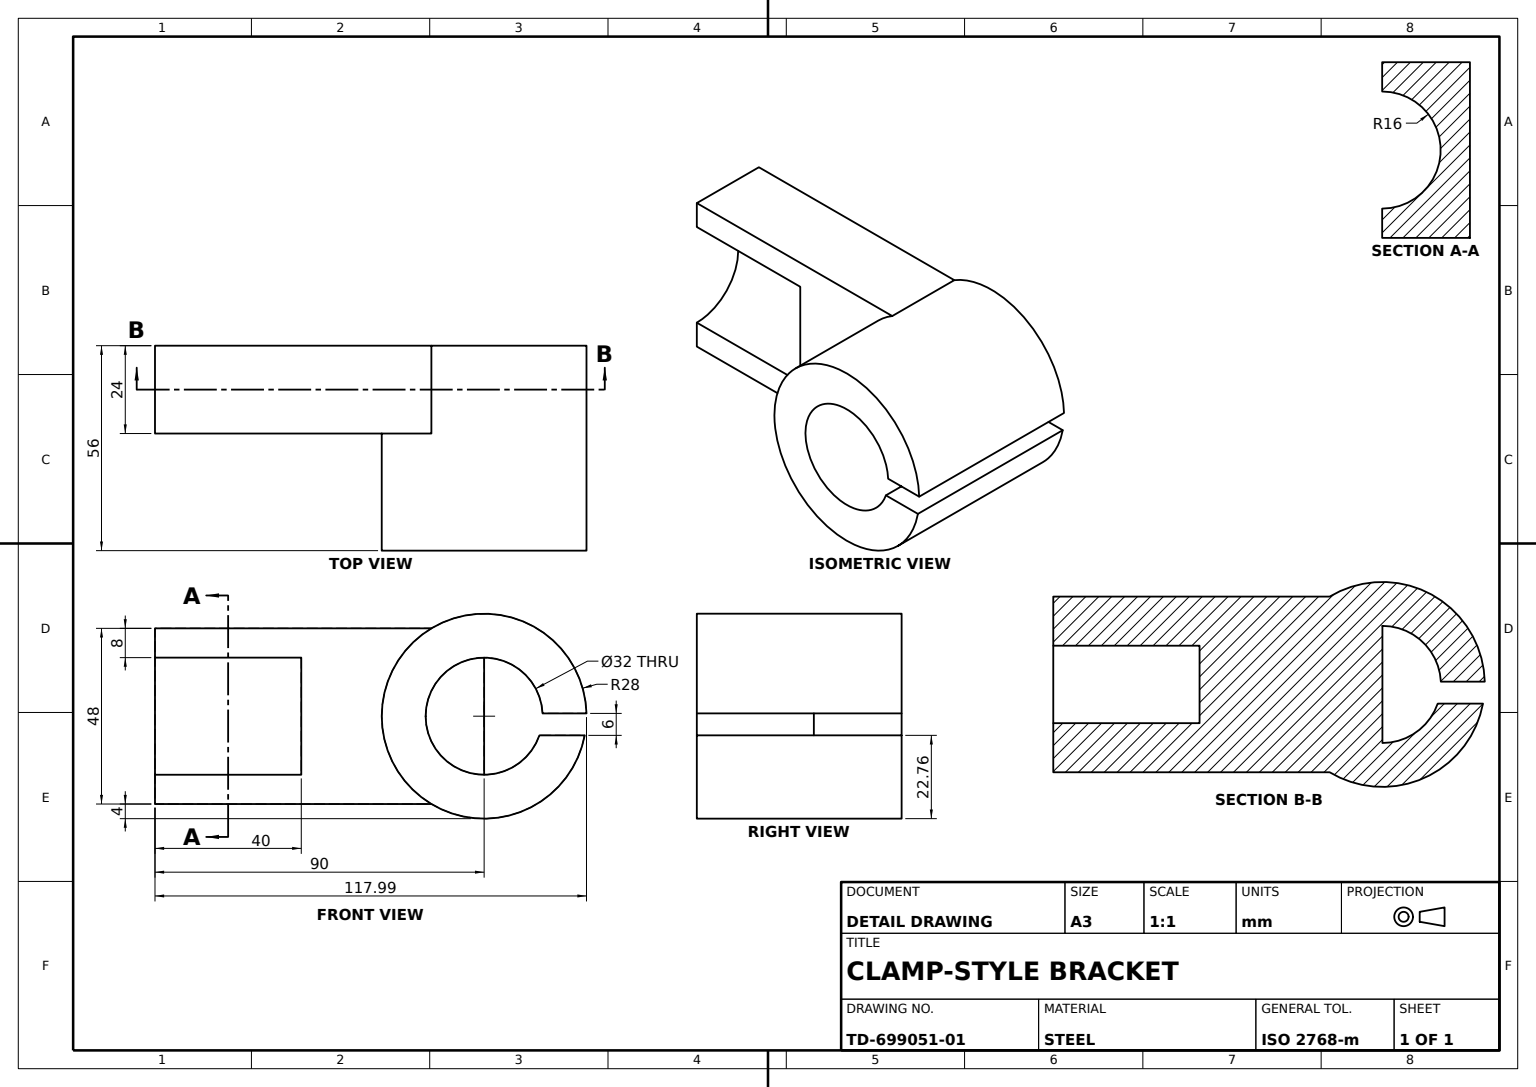
from build123d import *

# Parameters (mm, degrees)
BASE_BLOCK_SKETCH_W           = 90
BASE_BLOCK_SKETCH_H           = 48
BASE_BLOCK_DEPTH              = 12
CRADLE_CUT_DEPTH              = 40
CLAMP_BOSS_SKETCH_R           = 28
CLAMP_BOSS_SKETCH_R_2         = 16
CLAMP_BOSS_56_DEPTH           = 56
BORE_AND_SPLIT_SLOT_CUT_DEPTH = 56


with BuildPart() as part:
    # Base Block Sketch → Base Block (new, symmetric)
    with BuildSketch(Plane.XY):
        Rectangle(BASE_BLOCK_SKETCH_W, BASE_BLOCK_SKETCH_H)
    extrude(amount=BASE_BLOCK_DEPTH, both=True)

    # Cradle Cut Sketch → Cradle Cut (cut)
    with BuildSketch(Plane.ZY.offset(45)):
        with BuildLine():
            Line((12, -16), (12, 16))
            ThreePointArc((12, 16), (-4, 0), (12, -16))
        make_face()
    extrude(amount=-CRADLE_CUT_DEPTH, mode=Mode.SUBTRACT)

    # Clamp Boss Sketch → Clamp Boss Ø56 (add)
    with BuildSketch(Plane(origin=(0, 0, -12), x_dir=(-1, 0, 0), z_dir=(0, 0, -1))):
        with Locations((-45, 0)):
            Circle(CLAMP_BOSS_SKETCH_R)
        with Locations((-45, 0)):
            Circle(CLAMP_BOSS_SKETCH_R_2, mode=Mode.SUBTRACT)
    extrude(amount=-CLAMP_BOSS_56_DEPTH)

    # Bore and Split Slot Sketch → Bore and Split Slot Cut (cut)
    with BuildSketch(Plane.XY.offset(44)):
        Polygon((57.677488521, -2.241298623), (57.677488521, 0.758701377), (76.626798925, 0.758701377), (76.626798925, -5.241298623), (57.677488521, -5.241298623), align=None)
    extrude(amount=-BORE_AND_SPLIT_SLOT_CUT_DEPTH, mode=Mode.SUBTRACT)


solid = part.part
